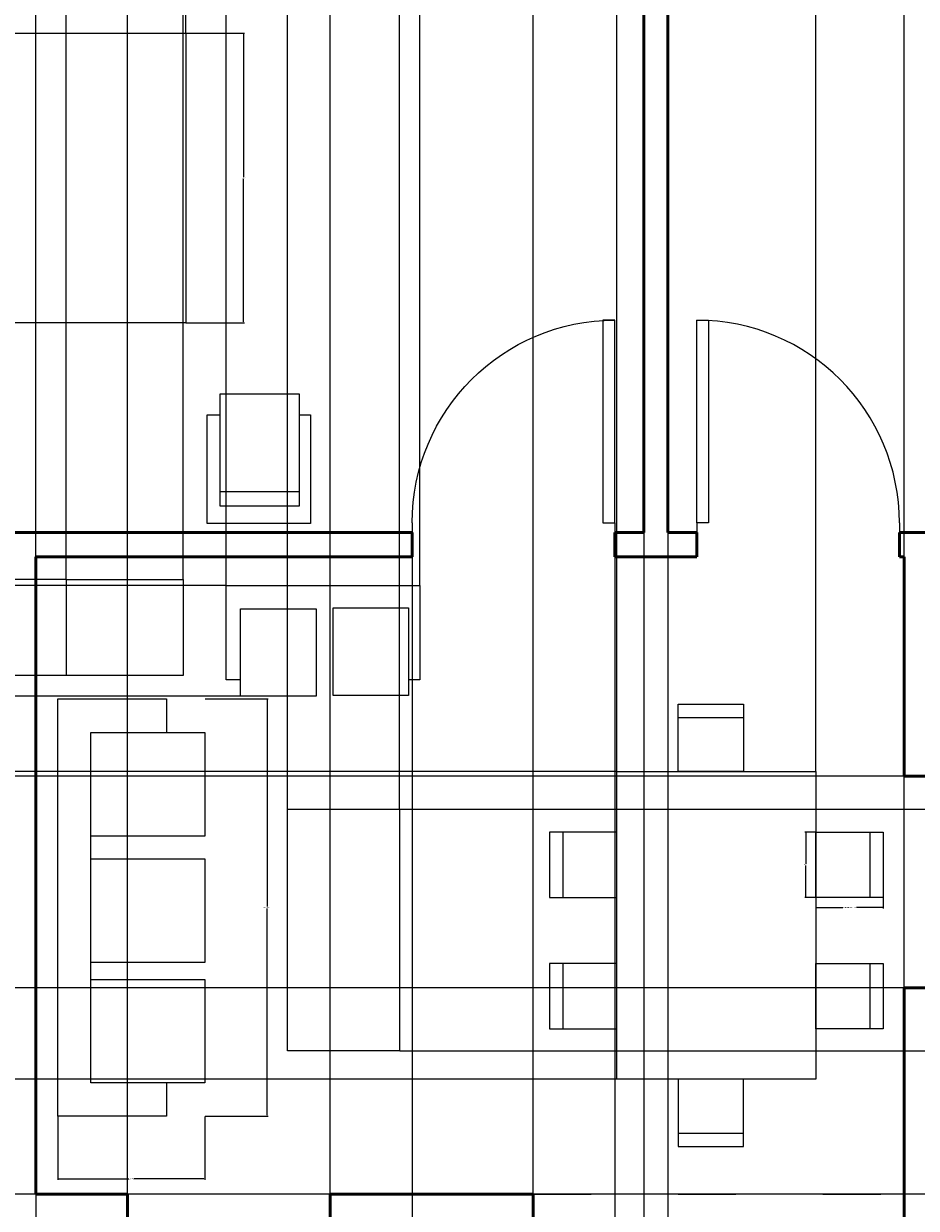
# Model space of a CAD drawing. Units: inches. Extents: x 115999 to 116502, y 188991 to 189729.
# Tile 3 of 5: x 116144 to 116329, y 189347 to 189592. Entities that reach past the tile are written whole.
import ezdxf

# ---------------------------------------------------------------- set-up
doc = ezdxf.new("R2010")
doc.units = ezdxf.units.IN
doc.linetypes.add('ACAD_ISO02W100', pattern=[15, 12, -3])
doc.linetypes.add('ACAD_ISO03W100', pattern=[30, 12, -18])
for name, color, linetype, lineweight in [('A-ANNO-DIMS', 2, 'Continuous', 18), ('A-DOOR', 4, 'Continuous', 25), ('A-FURN', 8, 'Continuous', 18), ('A-WALL', 7, 'Continuous', 50), ('A-WALL-OPEN', 7, 'ACAD_ISO03W100', 18), ('A-WALL-OVHD', 7, 'ACAD_ISO02W100', 18)]:
    doc.layers.add(name, color=color, linetype=linetype, lineweight=lineweight)
doc.styles.get("Standard").update_dxf_attribs({"font": 'arial.ttf'})
doc.dimstyles.get("Standard").update_dxf_attribs({"dimtxt": 0.18, "dimasz": 0.18, "dimexe": 0.18, "dimexo": 0.0625, "dimgap": 0.09, "dimtad": 0, "dimtih": 1, "dimtoh": 1, "dimdec": 4, "dimzin": 0, "dimdsep": 46, "dimtxsty": 'Standard', "dimcen": 0.09, "dimadec": 0, "dimazin": 0, "dimtfac": 1, "dimtdec": 4, "dimtofl": 0, "dimtmove": 0, "dimatfit": 3, "dimfxl": 1, "dimtolj": 1, "dimtzin": 0, "dimarcsym": 0})

# ---------------------------------------------------------------- blocks, each defined once
blk = doc.blocks.new('*U3')
for p, q in [((0, 0), (0, -5)), ((30, 0), (30, -5))]:
    blk.add_line(p, q)
blk.add_lwpolyline([(0, 0), (0, 30), (1.75, 30), (1.75, 0)], close=True)
blk.add_arc((0, 0), 30, 0, 90)
blk = doc.blocks.new('Bed - Queen')
for p, q in [((0, -80.00003), (0, 0)), ((0, 0), (59.99999, 0)), ((59.99999, 0), (59.99999, -80.00003)), ((7.99999, -1.2), (28.79998, -1.2)), ((7.99999, -14.4), (7.99999, -1.2)), ((28.79998, -1.2), (28.79998, -14.4)), ((31.19999, -1.2), (51.99999, -1.2)), ((31.19999, -14.4), (31.19999, -1.2)), ((51.99999, -1.2), (51.99999, -16.4)), ((0, -14.4), (44.8, -14.4)), ((59.99999, -29.6), (44.8, -14.4)), ((44.8, -14.4), (44.8, -29.6)), ((44.8, -16.8), (0, -16.8)), ((51.99999, -16.4), (46.79936, -16.4)), ((44.8, -29.6), (59.99999, -29.6)), ((59.99999, -80.00003), (0, -80.00003))]:
    blk.add_line(p, q)
blk = doc.blocks.new('SOFA-3-SEAT')
for points in [[(22.47, 6.88), (22.47, 0), (0, 0), (0, 86.44), (22.47, 86.44), (22.47, 79.43)], [(29.89, 6.88), (6.84, 6.88), (6.84, 79.43), (29.89, 79.43)]]:
    blk.add_lwpolyline(points)
for points in [[(30.42, 57.99), (6.84, 57.99), (6.84, 79.43), (30.42, 79.43)], [(30.42, 31.86), (6.84, 31.86), (6.84, 53.3), (30.42, 53.3)], [(30.42, 6.88), (6.84, 6.88), (6.84, 28.33), (30.42, 28.33)]]:
    blk.add_lwpolyline(points, close=True)
blk = doc.blocks.new('CHAIR-DINING')
blk.add_line((0, 11.19), (13.53, 11.19))
blk.add_lwpolyline([(0, 13.95), (13.53, 13.95), (13.53, 0), (0, 0)], close=True)
blk = doc.blocks.new('CHAIR-ARM')
blk.add_line((2.71, 6.64), (19.06, 6.64))
blk.add_lwpolyline([(2.71, 26.84), (19.06, 26.84), (19.06, 3.59), (2.71, 3.59)], close=True)
blk.add_lwpolyline([(19.06, 22.51), (21.46, 22.51), (21.46, 0), (0, 0), (0, 22.51), (2.71, 22.51)])
blk = doc.blocks.new('*D15')
at = {"layer": 'A-ANNO-DIMS', "color": 0, "lineweight": -2, "transparency": 16777216}
for p, q in [((116307.76, 189411.34), (116307.76, 189409.13)), ((116307.94, 189409.31), (116313.31, 189409.31)), ((116321.53, 189409.31), (116316.16, 189409.31)), ((116321.71, 189411.34), (116321.71, 189409.13))]:
    blk.add_line(p, q, dxfattribs=at)
at = {"layer": 'A-ANNO-DIMS', "color": 0, "transparency": 16777216}
for points in [[(116307.94, 189409.34), (116307.94, 189409.28), (116307.76, 189409.31)], [(116321.53, 189409.34), (116321.53, 189409.28), (116321.71, 189409.31)]]:
    blk.add_solid(points, dxfattribs=at)
at = {"layer": 'Defpoints', "color": 0, "transparency": 16777216}
for p in [(116307.76, 189411.41), (116321.71, 189411.41), (116321.71, 189409.31)]:
    blk.add_point(p, dxfattribs=at)
at = {"layer": 'A-ANNO-DIMS', "color": 0, "transparency": 16777216, "insert": (116314.74, 189409.31), "char_height": 0.18, "attachment_point": 5}
blk.add_mtext('\\A1;DINING CHAIR 14 TYP.', dxfattribs=at)
blk = doc.blocks.new('*D16')
at = {"layer": 'A-ANNO-DIMS', "color": 0, "lineweight": -2, "transparency": 16777216}
for p, q in [((116307.7, 189424.94), (116305.49, 189424.94)), ((116305.67, 189424.76), (116305.67, 189418.35)), ((116305.67, 189411.59), (116305.67, 189417.99)), ((116307.7, 189411.41), (116305.49, 189411.41))]:
    blk.add_line(p, q, dxfattribs=at)
at = {"layer": 'A-ANNO-DIMS', "color": 0, "transparency": 16777216}
for points in [[(116305.64, 189424.76), (116305.7, 189424.76), (116305.67, 189424.94)], [(116305.64, 189411.59), (116305.7, 189411.59), (116305.67, 189411.41)]]:
    blk.add_solid(points, dxfattribs=at)
at = {"layer": 'Defpoints', "color": 0, "transparency": 16777216}
for p in [(116307.76, 189424.94), (116305.67, 189411.41), (116307.76, 189411.41)]:
    blk.add_point(p, dxfattribs=at)
at = {"layer": 'A-ANNO-DIMS', "color": 0, "transparency": 16777216, "insert": (116305.67, 189418.17), "char_height": 0.18, "attachment_point": 5}
blk.add_mtext('\\A1;14 TYP.', dxfattribs=at)
blk = doc.blocks.new('*D21')
at = {"layer": 'A-ANNO-DIMS', "color": 0, "lineweight": -2, "transparency": 16777216}
for p, q in [((116097.14, 189590.46), (116097.14, 189602.58)), ((116097.32, 189602.4), (116135.84, 189602.4)), ((116176.96, 189602.4), (116138.45, 189602.4)), ((116177.14, 189590.46), (116177.14, 189602.58))]:
    blk.add_line(p, q, dxfattribs=at)
at = {"layer": 'A-ANNO-DIMS', "color": 0, "transparency": 16777216}
for points in [[(116097.32, 189602.43), (116097.32, 189602.37), (116097.14, 189602.4)], [(116176.96, 189602.43), (116176.96, 189602.37), (116177.14, 189602.4)]]:
    blk.add_solid(points, dxfattribs=at)
at = {"layer": 'Defpoints', "color": 0, "transparency": 16777216}
for p in [(116097.14, 189602.4), (116097.14, 189590.4), (116177.14, 189590.4)]:
    blk.add_point(p, dxfattribs=at)
at = {"layer": 'A-ANNO-DIMS', "color": 0, "transparency": 16777216, "insert": (116137.14, 189602.4), "char_height": 0.18, "attachment_point": 5}
blk.add_mtext('\\A1;QUEEN BED 80 TYP.', dxfattribs=at)
blk = doc.blocks.new('*D22')
at = {"layer": 'A-ANNO-DIMS', "color": 0, "lineweight": -2, "transparency": 16777216}
for p, q in [((116177.2, 189590.4), (116189.32, 189590.4)), ((116189.14, 189590.22), (116189.14, 189560.58)), ((116189.14, 189530.58), (116189.14, 189560.22)), ((116177.2, 189530.4), (116189.32, 189530.4))]:
    blk.add_line(p, q, dxfattribs=at)
at = {"layer": 'A-ANNO-DIMS', "color": 0, "transparency": 16777216}
for points in [[(116189.11, 189590.22), (116189.17, 189590.22), (116189.14, 189590.4)], [(116189.11, 189530.58), (116189.17, 189530.58), (116189.14, 189530.4)]]:
    blk.add_solid(points, dxfattribs=at)
at = {"layer": 'Defpoints', "color": 0, "transparency": 16777216}
for p in [(116177.14, 189590.4), (116189.14, 189590.4), (116177.14, 189530.4)]:
    blk.add_point(p, dxfattribs=at)
at = {"layer": 'A-ANNO-DIMS', "color": 0, "transparency": 16777216, "insert": (116189.14, 189560.4), "char_height": 0.18, "attachment_point": 5}
blk.add_mtext('\\A1;60 TYP.', dxfattribs=at)
blk = doc.blocks.new('*D25')
at = {"layer": 'A-ANNO-DIMS', "color": 0, "lineweight": -2, "transparency": 16777216}
for p, q in [((116181.15, 189452.53), (116194.23, 189452.53)), ((116194.05, 189452.35), (116194.05, 189409.49)), ((116194.05, 189366.27), (116194.05, 189409.13)), ((116181.15, 189366.09), (116194.23, 189366.09))]:
    blk.add_line(p, q, dxfattribs=at)
at = {"layer": 'A-ANNO-DIMS', "color": 0, "transparency": 16777216}
for points in [[(116194.02, 189452.35), (116194.08, 189452.35), (116194.05, 189452.53)], [(116194.02, 189366.27), (116194.08, 189366.27), (116194.05, 189366.09)]]:
    blk.add_solid(points, dxfattribs=at)
at = {"layer": 'Defpoints', "color": 0, "transparency": 16777216}
for p in [(116181.08, 189452.53), (116194.05, 189452.53), (116181.08, 189366.09)]:
    blk.add_point(p, dxfattribs=at)
at = {"layer": 'A-ANNO-DIMS', "color": 0, "transparency": 16777216, "insert": (116194.05, 189409.31), "char_height": 0.18, "attachment_point": 5}
blk.add_mtext('\\A1;SOFA 86 TYP.', dxfattribs=at)
blk = doc.blocks.new('*D26')
at = {"layer": 'A-ANNO-DIMS', "color": 0, "lineweight": -2, "transparency": 16777216}
for p, q in [((116150.66, 189366.03), (116150.66, 189352.94)), ((116181.08, 189366.03), (116181.08, 189352.94)), ((116150.84, 189353.12), (116165.34, 189353.12)), ((116180.9, 189353.12), (116166.4, 189353.12))]:
    blk.add_line(p, q, dxfattribs=at)
at = {"layer": 'A-ANNO-DIMS', "color": 0, "transparency": 16777216}
for points in [[(116150.84, 189353.15), (116150.84, 189353.09), (116150.66, 189353.12)], [(116180.9, 189353.15), (116180.9, 189353.09), (116181.08, 189353.12)]]:
    blk.add_solid(points, dxfattribs=at)
at = {"layer": 'Defpoints', "color": 0, "transparency": 16777216}
for p in [(116150.66, 189366.09), (116181.08, 189366.09), (116181.08, 189353.12)]:
    blk.add_point(p, dxfattribs=at)
at = {"layer": 'A-ANNO-DIMS', "color": 0, "transparency": 16777216, "insert": (116165.87, 189353.12), "char_height": 0.18, "attachment_point": 5}
blk.add_mtext('\\A1;30 TYP.', dxfattribs=at)
blk = doc.blocks.new('*D33')
at = {"layer": 'A-ANNO-DIMS', "color": 0, "lineweight": -2, "transparency": 16777216}
for p, q in [((116088.06, 189088.01), (116088.06, 189728.73)), ((116088.24, 189728.55), (116277.77, 189728.55)), ((116467.88, 189728.55), (116278.35, 189728.55)), ((116468.06, 189088.01), (116468.06, 189728.73))]:
    blk.add_line(p, q, dxfattribs=at)
at = {"layer": 'A-ANNO-DIMS', "color": 0, "transparency": 16777216}
for points in [[(116088.24, 189728.58), (116088.24, 189728.52), (116088.06, 189728.55)], [(116467.88, 189728.58), (116467.88, 189728.52), (116468.06, 189728.55)]]:
    blk.add_solid(points, dxfattribs=at)
at = {"layer": 'Defpoints', "color": 0, "transparency": 16777216}
for p in [(116468.06, 189728.55), (116088.06, 189087.95), (116468.06, 189087.95)]:
    blk.add_point(p, dxfattribs=at)
at = {"layer": 'A-ANNO-DIMS', "color": 0, "transparency": 16777216, "insert": (116278.06, 189728.55), "char_height": 0.18, "attachment_point": 5}
blk.add_mtext('\\A1;380', dxfattribs=at)
blk = doc.blocks.new('*D43')
at = {"layer": 'A-ANNO-DIMS', "color": 0, "lineweight": -2, "transparency": 16777216}
for p, q in [((116093.06, 189624.88), (116093.06, 188991.26)), ((116272.06, 189624.88), (116272.06, 188991.26)), ((116093.24, 188991.44), (116182.28, 188991.44)), ((116271.88, 188991.44), (116182.84, 188991.44))]:
    blk.add_line(p, q, dxfattribs=at)
at = {"layer": 'A-ANNO-DIMS', "color": 0, "transparency": 16777216}
for points in [[(116093.24, 188991.47), (116093.24, 188991.41), (116093.06, 188991.44)], [(116271.88, 188991.47), (116271.88, 188991.41), (116272.06, 188991.44)]]:
    blk.add_solid(points, dxfattribs=at)
at = {"layer": 'Defpoints', "color": 0, "transparency": 16777216}
for p in [(116093.06, 189624.95), (116272.06, 189624.95), (116272.06, 188991.44)]:
    blk.add_point(p, dxfattribs=at)
at = {"layer": 'A-ANNO-DIMS', "color": 0, "transparency": 16777216, "insert": (116182.56, 188991.44), "char_height": 0.18, "attachment_point": 5}
blk.add_mtext('\\A1;179', dxfattribs=at)
blk = doc.blocks.new('*D44')
at = {"layer": 'A-ANNO-DIMS', "color": 0, "lineweight": -2, "transparency": 16777216}
for p, q in [((116277.06, 189624.88), (116277.06, 188991.26)), ((116463.06, 189624.88), (116463.06, 188991.26)), ((116277.24, 188991.44), (116369.78, 188991.44)), ((116462.88, 188991.44), (116370.34, 188991.44))]:
    blk.add_line(p, q, dxfattribs=at)
at = {"layer": 'A-ANNO-DIMS', "color": 0, "transparency": 16777216}
for points in [[(116277.24, 188991.47), (116277.24, 188991.41), (116277.06, 188991.44)], [(116462.88, 188991.47), (116462.88, 188991.41), (116463.06, 188991.44)]]:
    blk.add_solid(points, dxfattribs=at)
at = {"layer": 'Defpoints', "color": 0, "transparency": 16777216}
for p in [(116277.06, 189624.95), (116463.06, 189624.95), (116463.06, 188991.44)]:
    blk.add_point(p, dxfattribs=at)
at = {"layer": 'A-ANNO-DIMS', "color": 0, "transparency": 16777216, "insert": (116370.06, 188991.44), "char_height": 0.18, "attachment_point": 5}
blk.add_mtext('\\A1;186', dxfattribs=at)
blk = doc.blocks.new('*D45')
at = {"layer": 'A-ANNO-DIMS', "color": 0, "lineweight": -2, "transparency": 16777216}
for p, q in [((116272.06, 189624.88), (116272.06, 188991.26)), ((116277.06, 189624.88), (116277.06, 188991.26)), ((116272.24, 188991.44), (116274.41, 188991.44)), ((116276.88, 188991.44), (116274.71, 188991.44))]:
    blk.add_line(p, q, dxfattribs=at)
at = {"layer": 'A-ANNO-DIMS', "color": 0, "transparency": 16777216}
for points in [[(116272.24, 188991.47), (116272.24, 188991.41), (116272.06, 188991.44)], [(116276.88, 188991.47), (116276.88, 188991.41), (116277.06, 188991.44)]]:
    blk.add_solid(points, dxfattribs=at)
at = {"layer": 'Defpoints', "color": 0, "transparency": 16777216}
for p in [(116272.06, 189624.95), (116277.06, 189624.95), (116277.06, 188991.44)]:
    blk.add_point(p, dxfattribs=at)
at = {"layer": 'A-ANNO-DIMS', "color": 0, "transparency": 16777216, "insert": (116274.56, 188991.44), "char_height": 0.18, "attachment_point": 5}
blk.add_mtext('\\A1;5', dxfattribs=at)
blk = doc.blocks.new('*D46')
at = {"layer": 'A-ANNO-DIMS', "color": 0, "lineweight": -2, "transparency": 16777216}
for p, q in [((116224.06, 189486.88), (116224.06, 188991.26)), ((116266.06, 189486.88), (116266.06, 188991.26)), ((116224.24, 188991.44), (116244.84, 188991.44)), ((116265.88, 188991.44), (116245.28, 188991.44))]:
    blk.add_line(p, q, dxfattribs=at)
at = {"layer": 'A-ANNO-DIMS', "color": 0, "transparency": 16777216}
for points in [[(116224.24, 188991.47), (116224.24, 188991.41), (116224.06, 188991.44)], [(116265.88, 188991.47), (116265.88, 188991.41), (116266.06, 188991.44)]]:
    blk.add_solid(points, dxfattribs=at)
at = {"layer": 'Defpoints', "color": 0, "transparency": 16777216}
for p in [(116224.06, 189486.95), (116266.06, 189486.95), (116266.06, 188991.44)]:
    blk.add_point(p, dxfattribs=at)
at = {"layer": 'A-ANNO-DIMS', "color": 0, "transparency": 16777216, "insert": (116245.06, 188991.44), "char_height": 0.18, "attachment_point": 5}
blk.add_mtext('\\A1;42', dxfattribs=at)
blk = doc.blocks.new('*D47')
at = {"layer": 'A-ANNO-DIMS', "color": 0, "lineweight": -2, "transparency": 16777216}
for p, q in [((116266.063078, 189486.884428), (116266.063078, 188991.259265)), ((116272.063078, 189486.884428), (116272.063078, 188991.259265)), ((116266.243078, 188991.439265), (116268.913651, 188991.439265)), ((116271.883078, 188991.439265), (116269.212505, 188991.439265))]:
    blk.add_line(p, q, dxfattribs=at)
at = {"layer": 'A-ANNO-DIMS', "color": 0, "transparency": 16777216}
for points in [[(116266.243078, 188991.469265), (116266.243078, 188991.409265), (116266.063078, 188991.439265)], [(116271.883078, 188991.469265), (116271.883078, 188991.409265), (116272.063078, 188991.439265)]]:
    blk.add_solid(points, dxfattribs=at)
at = {"layer": 'Defpoints', "color": 0, "transparency": 16777216}
for p in [(116266.063078, 189486.946928), (116272.063078, 189486.946928), (116272.063078, 188991.439265)]:
    blk.add_point(p, dxfattribs=at)
at = {"layer": 'A-ANNO-DIMS', "color": 0, "transparency": 16777216, "insert": (116269.063078, 188991.439265), "char_height": 0.18, "attachment_point": 5}
blk.add_mtext('\\A1;6', dxfattribs=at)
blk = doc.blocks.new('*D50')
at = {"layer": 'A-ANNO-DIMS', "color": 0, "lineweight": -2, "transparency": 16777216}
for p, q in [((116146.06, 189349.88), (116146.06, 188991.26)), ((116326.06, 189349.88), (116326.06, 188991.26)), ((116146.24, 188991.44), (116235.78, 188991.44)), ((116325.88, 188991.44), (116236.34, 188991.44))]:
    blk.add_line(p, q, dxfattribs=at)
at = {"layer": 'A-ANNO-DIMS', "color": 0, "transparency": 16777216}
for points in [[(116146.24, 188991.47), (116146.24, 188991.41), (116146.06, 188991.44)], [(116325.88, 188991.47), (116325.88, 188991.41), (116326.06, 188991.44)]]:
    blk.add_solid(points, dxfattribs=at)
at = {"layer": 'Defpoints', "color": 0, "transparency": 16777216}
for p in [(116146.06, 189349.95), (116326.06, 189349.95), (116326.06, 188991.44)]:
    blk.add_point(p, dxfattribs=at)
at = {"layer": 'A-ANNO-DIMS', "color": 0, "transparency": 16777216, "insert": (116236.06, 188991.44), "char_height": 0.18, "attachment_point": 5}
blk.add_mtext('\\A1;180', dxfattribs=at)
blk = doc.blocks.new('*D53')
at = {"layer": 'A-ANNO-DIMS', "color": 0, "lineweight": -2, "transparency": 16777216}
for p, q in [((116331, 189436.5), (115999.04, 189436.5)), ((115999.22, 189436.32), (115999.22, 189414.77)), ((115999.22, 189392.85), (115999.22, 189414.41)), ((116331, 189392.67), (115999.04, 189392.67))]:
    blk.add_line(p, q, dxfattribs=at)
at = {"layer": 'A-ANNO-DIMS', "color": 0, "transparency": 16777216}
for points in [[(115999.19, 189436.32), (115999.25, 189436.32), (115999.22, 189436.5)], [(115999.19, 189392.85), (115999.25, 189392.85), (115999.22, 189392.67)]]:
    blk.add_solid(points, dxfattribs=at)
at = {"layer": 'Defpoints', "color": 0, "transparency": 16777216}
for p in [(115999.22, 189436.5), (116331.06, 189436.5), (116331.06, 189392.67)]:
    blk.add_point(p, dxfattribs=at)
at = {"layer": 'A-ANNO-DIMS', "color": 0, "transparency": 16777216, "insert": (115999.22, 189414.59), "char_height": 0.18, "attachment_point": 5}
blk.add_mtext('\\A1;43.83', dxfattribs=at)
blk = doc.blocks.new('*D54')
at = {"layer": 'A-ANNO-DIMS', "color": 0, "lineweight": -2, "transparency": 16777216}
for p, q in [((116266.5, 189437.51), (116266.5, 189728.73)), ((116266.68, 189728.55), (116286.73, 189728.55)), ((116307.58, 189728.55), (116287.53, 189728.55)), ((116307.76, 189437.51), (116307.76, 189728.73))]:
    blk.add_line(p, q, dxfattribs=at)
at = {"layer": 'A-ANNO-DIMS', "color": 0, "transparency": 16777216}
for points in [[(116266.68, 189728.58), (116266.68, 189728.52), (116266.5, 189728.55)], [(116307.58, 189728.58), (116307.58, 189728.52), (116307.76, 189728.55)]]:
    blk.add_solid(points, dxfattribs=at)
at = {"layer": 'Defpoints', "color": 0, "transparency": 16777216}
for p in [(116307.76, 189728.55), (116266.5, 189437.45), (116307.76, 189437.45)]:
    blk.add_point(p, dxfattribs=at)
at = {"layer": 'A-ANNO-DIMS', "color": 0, "transparency": 16777216, "insert": (116287.13, 189728.55), "char_height": 0.18, "attachment_point": 5}
blk.add_mtext('\\A1;41.26', dxfattribs=at)
blk = doc.blocks.new('*D55')
at = {"layer": 'A-ANNO-DIMS', "color": 0, "lineweight": -2, "transparency": 16777216}
for p, q in [((116266.44, 189437.45), (115999.04, 189437.45)), ((115999.22, 189437.27), (115999.22, 189405.79)), ((115999.22, 189373.95), (115999.22, 189405.43)), ((116266.44, 189373.77), (115999.04, 189373.77))]:
    blk.add_line(p, q, dxfattribs=at)
at = {"layer": 'A-ANNO-DIMS', "color": 0, "transparency": 16777216}
for points in [[(115999.19, 189437.27), (115999.25, 189437.27), (115999.22, 189437.45)], [(115999.19, 189373.95), (115999.25, 189373.95), (115999.22, 189373.77)]]:
    blk.add_solid(points, dxfattribs=at)
at = {"layer": 'Defpoints', "color": 0, "transparency": 16777216}
for p in [(115999.22, 189437.45), (116266.5, 189437.45), (116266.5, 189373.77)]:
    blk.add_point(p, dxfattribs=at)
at = {"layer": 'A-ANNO-DIMS', "color": 0, "transparency": 16777216, "insert": (115999.22, 189405.61), "char_height": 0.18, "attachment_point": 5}
blk.add_mtext('\\A1;63.68', dxfattribs=at)
blk = doc.blocks.new('*D67')
at = {"layer": 'A-ANNO-DIMS', "color": 0, "lineweight": -2, "transparency": 16777216}
for p, q in [((116331, 189392.67), (115999.04, 189392.67)), ((115999.22, 189392.49), (115999.22, 189371.49)), ((115999.22, 189350.13), (115999.22, 189371.13)), ((116331, 189349.95), (115999.04, 189349.95))]:
    blk.add_line(p, q, dxfattribs=at)
at = {"layer": 'A-ANNO-DIMS', "color": 0, "transparency": 16777216}
for points in [[(115999.19, 189392.49), (115999.25, 189392.49), (115999.22, 189392.67)], [(115999.19, 189350.13), (115999.25, 189350.13), (115999.22, 189349.95)]]:
    blk.add_solid(points, dxfattribs=at)
at = {"layer": 'Defpoints', "color": 0, "transparency": 16777216}
for p in [(115999.22, 189392.67), (116331.06, 189392.67), (116331.06, 189349.95)]:
    blk.add_point(p, dxfattribs=at)
at = {"layer": 'A-ANNO-DIMS', "color": 0, "transparency": 16777216, "insert": (115999.22, 189371.31), "char_height": 0.18, "attachment_point": 5}
blk.add_mtext('\\A1;42.73', dxfattribs=at)
blk = doc.blocks.new('*D71')
at = {"layer": 'A-ANNO-DIMS', "color": 0, "lineweight": -2, "transparency": 16777216}
for p, q in [((116165.06, 189350.01), (116165.06, 189728.73)), ((116165.24, 189728.55), (116185.84, 189728.55)), ((116206.88, 189728.55), (116186.28, 189728.55)), ((116207.06, 189350.01), (116207.06, 189728.73))]:
    blk.add_line(p, q, dxfattribs=at)
at = {"layer": 'A-ANNO-DIMS', "color": 0, "transparency": 16777216}
for points in [[(116165.24, 189728.58), (116165.24, 189728.52), (116165.06, 189728.55)], [(116206.88, 189728.58), (116206.88, 189728.52), (116207.06, 189728.55)]]:
    blk.add_solid(points, dxfattribs=at)
at = {"layer": 'Defpoints', "color": 0, "transparency": 16777216}
for p in [(116207.06, 189728.55), (116165.06, 189349.95), (116207.06, 189349.95)]:
    blk.add_point(p, dxfattribs=at)
at = {"layer": 'A-ANNO-DIMS', "color": 0, "transparency": 16777216, "insert": (116186.06, 189728.55), "char_height": 0.18, "attachment_point": 5}
blk.add_mtext('\\A1;42', dxfattribs=at)
blk = doc.blocks.new('*D72')
at = {"layer": 'A-ANNO-DIMS', "color": 0, "lineweight": -2, "transparency": 16777216}
for p, q in [((116249.18, 189350.01), (116249.18, 189728.73)), ((116249.36, 189728.55), (116287.23, 189728.55)), ((116325.88, 189728.55), (116288.02, 189728.55)), ((116326.06, 189350.01), (116326.06, 189728.73))]:
    blk.add_line(p, q, dxfattribs=at)
at = {"layer": 'A-ANNO-DIMS', "color": 0, "transparency": 16777216}
for points in [[(116249.36, 189728.58), (116249.36, 189728.52), (116249.18, 189728.55)], [(116325.88, 189728.58), (116325.88, 189728.52), (116326.06, 189728.55)]]:
    blk.add_solid(points, dxfattribs=at)
at = {"layer": 'Defpoints', "color": 0, "transparency": 16777216}
for p in [(116326.06, 189728.55), (116249.18, 189349.95), (116326.06, 189349.95)]:
    blk.add_point(p, dxfattribs=at)
at = {"layer": 'A-ANNO-DIMS', "color": 0, "transparency": 16777216, "insert": (116287.62, 189728.55), "char_height": 0.18, "attachment_point": 5}
blk.add_mtext('\\A1;76.88', dxfattribs=at)
blk = doc.blocks.new('*D74')
at = {"layer": 'A-ANNO-DIMS', "color": 0, "lineweight": -2, "transparency": 16777216}
for p, q in [((116146.06, 189350.01), (116146.06, 189728.73)), ((116146.24, 189728.55), (116155.35, 189728.55)), ((116164.88, 189728.55), (116155.77, 189728.55)), ((116165.06, 189350.01), (116165.06, 189728.73))]:
    blk.add_line(p, q, dxfattribs=at)
at = {"layer": 'A-ANNO-DIMS', "color": 0, "transparency": 16777216}
for points in [[(116146.24, 189728.58), (116146.24, 189728.52), (116146.06, 189728.55)], [(116164.88, 189728.58), (116164.88, 189728.52), (116165.06, 189728.55)]]:
    blk.add_solid(points, dxfattribs=at)
at = {"layer": 'Defpoints', "color": 0, "transparency": 16777216}
for p in [(116165.06, 189728.55), (116146.06, 189349.95), (116165.06, 189349.95)]:
    blk.add_point(p, dxfattribs=at)
at = {"layer": 'A-ANNO-DIMS', "color": 0, "transparency": 16777216, "insert": (116155.56, 189728.55), "char_height": 0.18, "attachment_point": 5}
blk.add_mtext('\\A1;19', dxfattribs=at)
blk = doc.blocks.new('*D78')
at = {"layer": 'A-ANNO-DIMS', "color": 0, "lineweight": -2, "transparency": 16777216}
for p, q in [((116198.25, 189429.74), (116198.25, 189728.73)), ((116198.43, 189728.55), (116209.47, 189728.55)), ((116221.29, 189728.55), (116210.25, 189728.55)), ((116221.47, 189429.74), (116221.47, 189728.73))]:
    blk.add_line(p, q, dxfattribs=at)
at = {"layer": 'A-ANNO-DIMS', "color": 0, "transparency": 16777216}
for points in [[(116198.43, 189728.58), (116198.43, 189728.52), (116198.25, 189728.55)], [(116221.29, 189728.58), (116221.29, 189728.52), (116221.47, 189728.55)]]:
    blk.add_solid(points, dxfattribs=at)
at = {"layer": 'Defpoints', "color": 0, "transparency": 16777216}
for p in [(116221.47, 189728.55), (116198.25, 189429.68), (116221.47, 189429.68)]:
    blk.add_point(p, dxfattribs=at)
at = {"layer": 'A-ANNO-DIMS', "color": 0, "transparency": 16777216, "insert": (116209.86, 189728.55), "char_height": 0.18, "attachment_point": 5}
blk.add_mtext('\\A1;23.22', dxfattribs=at)
blk = doc.blocks.new('*D79')
at = {"layer": 'A-ANNO-DIMS', "color": 0, "lineweight": -2, "transparency": 16777216}
for p, q in [((116221.53, 189429.68), (116501.84, 189429.68)), ((116501.66, 189429.5), (116501.66, 189404.83)), ((116501.66, 189379.81), (116501.66, 189404.47)), ((116221.53, 189379.63), (116501.84, 189379.63))]:
    blk.add_line(p, q, dxfattribs=at)
at = {"layer": 'A-ANNO-DIMS', "color": 0, "transparency": 16777216}
for points in [[(116501.63, 189429.5), (116501.69, 189429.5), (116501.66, 189429.68)], [(116501.63, 189379.81), (116501.69, 189379.81), (116501.66, 189379.63)]]:
    blk.add_solid(points, dxfattribs=at)
at = {"layer": 'Defpoints', "color": 0, "transparency": 16777216}
for p in [(116221.47, 189429.68), (116501.66, 189429.68), (116221.47, 189379.63)]:
    blk.add_point(p, dxfattribs=at)
at = {"layer": 'A-ANNO-DIMS', "color": 0, "transparency": 16777216, "insert": (116501.66, 189404.65), "char_height": 0.18, "attachment_point": 5}
blk.add_mtext('\\A1;50.05', dxfattribs=at)
blk = doc.blocks.new('*D80')
at = {"layer": 'A-ANNO-DIMS', "color": 0, "lineweight": -2, "transparency": 16777216}
for p, q in [((116185.52, 189476.05), (116185.52, 189728.73)), ((116185.7, 189728.55), (116205.21, 189728.55)), ((116225.51, 189728.55), (116206, 189728.55)), ((116225.69, 189476.05), (116225.69, 189728.73))]:
    blk.add_line(p, q, dxfattribs=at)
at = {"layer": 'A-ANNO-DIMS', "color": 0, "transparency": 16777216}
for points in [[(116185.7, 189728.58), (116185.7, 189728.52), (116185.52, 189728.55)], [(116225.51, 189728.58), (116225.51, 189728.52), (116225.69, 189728.55)]]:
    blk.add_solid(points, dxfattribs=at)
at = {"layer": 'Defpoints', "color": 0, "transparency": 16777216}
for p in [(116225.69, 189728.55), (116185.52, 189475.99), (116225.69, 189475.99)]:
    blk.add_point(p, dxfattribs=at)
at = {"layer": 'A-ANNO-DIMS', "color": 0, "transparency": 16777216, "insert": (116205.6, 189728.55), "char_height": 0.18, "attachment_point": 5}
blk.add_mtext('\\A1;40.17', dxfattribs=at)
blk = doc.blocks.new('*D81')
at = {"layer": 'A-ANNO-DIMS', "color": 0, "lineweight": -2, "transparency": 16777216}
for p, q in [((116185.46, 189475.99), (115999.04, 189475.99)), ((115999.22, 189475.81), (115999.22, 189464.71)), ((115999.22, 189453.24), (115999.22, 189464.34)), ((116188.46, 189453.06), (115999.04, 189453.06))]:
    blk.add_line(p, q, dxfattribs=at)
at = {"layer": 'A-ANNO-DIMS', "color": 0, "transparency": 16777216}
for points in [[(115999.19, 189475.81), (115999.25, 189475.81), (115999.22, 189475.99)], [(115999.19, 189453.24), (115999.25, 189453.24), (115999.22, 189453.06)]]:
    blk.add_solid(points, dxfattribs=at)
at = {"layer": 'Defpoints', "color": 0, "transparency": 16777216}
for p in [(116185.52, 189475.99), (115999.22, 189453.06), (116188.52, 189453.06)]:
    blk.add_point(p, dxfattribs=at)
at = {"layer": 'A-ANNO-DIMS', "color": 0, "transparency": 16777216, "insert": (115999.22, 189464.52), "char_height": 0.18, "attachment_point": 5}
blk.add_mtext('\\A1;22.926', dxfattribs=at)
blk = doc.blocks.new('*D82')
at = {"layer": 'A-ANNO-DIMS', "color": 0, "lineweight": -2, "transparency": 16777216}
for p, q in [((116152.4, 189477.27), (116152.4, 189728.73)), ((116152.58, 189728.55), (116164.04, 189728.55)), ((116176.43, 189728.55), (116164.97, 189728.55)), ((116176.61, 189477.27), (116176.61, 189728.73))]:
    blk.add_line(p, q, dxfattribs=at)
at = {"layer": 'A-ANNO-DIMS', "color": 0, "transparency": 16777216}
for points in [[(116152.58, 189728.58), (116152.58, 189728.52), (116152.4, 189728.55)], [(116176.43, 189728.58), (116176.43, 189728.52), (116176.61, 189728.55)]]:
    blk.add_solid(points, dxfattribs=at)
at = {"layer": 'Defpoints', "color": 0, "transparency": 16777216}
for p in [(116176.61, 189728.55), (116152.4, 189477.21), (116176.61, 189477.21)]:
    blk.add_point(p, dxfattribs=at)
at = {"layer": 'A-ANNO-DIMS', "color": 0, "transparency": 16777216, "insert": (116164.51, 189728.55), "char_height": 0.18, "attachment_point": 5}
blk.add_mtext('\\A1;24.204', dxfattribs=at)
blk = doc.blocks.new('*D83')
at = {"layer": 'A-ANNO-DIMS', "color": 0, "lineweight": -2, "transparency": 16777216}
for p, q in [((116152.34, 189477.21), (115999.04, 189477.21)), ((115999.22, 189477.03), (115999.22, 189467.47)), ((115999.22, 189457.56), (115999.22, 189467.11)), ((116152.34, 189457.38), (115999.04, 189457.38))]:
    blk.add_line(p, q, dxfattribs=at)
at = {"layer": 'A-ANNO-DIMS', "color": 0, "transparency": 16777216}
for points in [[(115999.19, 189477.03), (115999.25, 189477.03), (115999.22, 189477.21)], [(115999.19, 189457.56), (115999.25, 189457.56), (115999.22, 189457.38)]]:
    blk.add_solid(points, dxfattribs=at)
at = {"layer": 'Defpoints', "color": 0, "transparency": 16777216}
for p in [(115999.22, 189477.21), (116152.4, 189477.21), (116152.4, 189457.38)]:
    blk.add_point(p, dxfattribs=at)
at = {"layer": 'A-ANNO-DIMS', "color": 0, "transparency": 16777216, "insert": (115999.22, 189467.29), "char_height": 0.18, "attachment_point": 5}
blk.add_mtext('\\A1;19.83', dxfattribs=at)

msp = doc.modelspace()

# ---------------------------------------------------------------- linework, layer by layer
at = {"layer": 'A-FURN'}
for points in [[(116152.4048, 189477.2058), (116176.6085, 189477.2058), (116176.6085, 189457.376), (116152.4048, 189457.376)], [(116188.5186, 189471.1941), (116204.1981, 189471.1941), (116204.1981, 189453.0603), (116188.5186, 189453.0603)], [(116207.6703, 189471.3815), (116223.3498, 189471.3815), (116223.3498, 189453.2476), (116207.6703, 189453.2476)], [(116266.5001, 189437.4482), (116307.7598, 189437.4482), (116307.7598, 189373.7675), (116266.5001, 189373.7675)], [(116198.2486, 189429.6768), (116221.4703, 189429.6768), (116221.4703, 189379.6257), (116198.2486, 189379.6257)]]:
    msp.add_lwpolyline(points, close=True, dxfattribs=at)
for points in [[(116188.5186, 189456.4441), (116185.5193, 189456.4441), (116185.5193, 189475.9866), (116225.6867, 189475.9866), (116225.6867, 189456.4441)], [(116225.6867, 189456.4441), (116223.3498, 189456.4441)]]:
    msp.add_lwpolyline(points, dxfattribs=at)
at = {"layer": 'A-WALL'}
for p, q in [((116272.0631, 189624.9469), (116272.0631, 189486.9469)), ((116277.0631, 189624.9469), (116277.0631, 189486.9469)), ((116093.0631, 189486.9469), (116224.0631, 189486.9469)), ((116224.0631, 189486.9469), (116224.0631, 189481.9469)), ((116266.0631, 189486.9469), (116266.0631, 189481.9469)), ((116266.0631, 189486.9469), (116272.0631, 189486.9469)), ((116277.0631, 189486.9469), (116283.0631, 189486.9469)), ((116283.0631, 189486.9469), (116283.0631, 189481.9469)), ((116325.0631, 189486.9469), (116325.0631, 189481.9469)), ((116325.0631, 189486.9469), (116463.0631, 189486.9469)), ((116146.0631, 189481.9469), (116146.0631, 189349.9469)), ((116146.0631, 189481.9469), (116224.0631, 189481.9469)), ((116266.0631, 189481.9469), (116283.0631, 189481.9469)), ((116277.0631, 189481.9469), (116283.0631, 189481.9469)), ((116325.0631, 189481.9469), (116326.0631, 189481.9469)), ((116325.0631, 189481.9469), (116326.0631, 189481.9469)), ((116326.0631, 189481.9469), (116326.0631, 189436.5016)), ((116326.0631, 189436.5016), (116331.0631, 189436.5016)), ((116326.0631, 189392.6745), (116331.0631, 189392.6745)), ((116326.0631, 189392.6745), (116326.0631, 189344.9469)), ((116146.0631, 189349.9469), (116165.0631, 189349.9469)), ((116165.0631, 189344.9469), (116165.0631, 189349.9469)), ((116207.0631, 189344.9469), (116207.0631, 189349.9469)), ((116207.0631, 189349.9469), (116249.1823, 189349.9469)), ((116249.1823, 189344.9469), (116249.1823, 189349.9469))]:
    msp.add_line(p, q, dxfattribs=at)
at = {"layer": 'A-WALL-OPEN'}
msp.add_line((116249.1823, 189349.9469), (116326.0631, 189349.9469), dxfattribs=at)
at = {"layer": 'A-WALL-OVHD'}
msp.add_line((116326.0631, 189392.6745), (116326.0631, 189436.5016), dxfattribs=at)

# ---------------------------------------------------------------- block references
at = {"layer": 'A-DOOR', "yscale": 1.400000000000193, "zscale": 1.400000000000193}
for p, xscale in [((116266.0631, 189488.9469), -1.400000000000193), ((116283.0631, 189488.9469), 1.400000000000193)]:
    msp.add_blockref('*U3', p, dxfattribs=dict(at, xscale=xscale))
at = {"layer": 'A-DOOR', "xscale": 1.400000000000193, "yscale": 1.400000000000193, "zscale": 1.400000000000193, "rotation": 180}
msp.add_blockref('*U3', (116207.0631, 189342.9469), dxfattribs=at)
at = {"layer": 'A-FURN'}
for name, p, rotation in [('Bed - Queen', (116097.142, 189530.3971), 90), ('CHAIR-DINING', (116307.7598, 189424.94), 269.9999999998937), ('CHAIR-DINING', (116307.7598, 189397.7046), 269.9999999998937)]:
    msp.add_blockref(name, p, dxfattribs=dict(at, rotation=rotation))
for name, p in [('CHAIR-ARM', (116181.5682, 189488.8569)), ('SOFA-3-SEAT', (116150.6627, 189366.0896)), ('CHAIR-DINING', (116279.2191, 189437.4482))]:
    msp.add_blockref(name, p, dxfattribs=at)
at = {"layer": 'A-FURN', "extrusion": (0, 0, -1), "zscale": -1}
for p, rotation in [((-116266.5001, 189424.94), 269.9999999998937), ((-116266.5001, 189397.7046), 269.9999999998937), ((-116279.2191, 189373.7675), 180)]:
    msp.add_blockref('CHAIR-DINING', p, dxfattribs=dict(at, rotation=rotation))

# ---------------------------------------------------------------- dimensions: what is measured, and where the dimension line sits
at = {"layer": 'A-ANNO-DIMS'}
for base, p1, p2, override, picture, middle in [((116468.0631, 189728.5469), (116088.0631, 189087.9469), (116468.0631, 189087.9469), {"dimdec": 0, "dimlfac": 1, "dimrnd": 0, "dimzin": 0, "dimdsep": 46, "dimlunit": 2}, '*D33', (116278.0631, 189728.5469)), ((116165.0631, 189728.5469), (116146.0631, 189349.9469), (116165.0631, 189349.9469), {"dimdec": 0, "dimlfac": 1, "dimrnd": 0, "dimzin": 0, "dimdsep": 46, "dimlunit": 2}, '*D74', (116155.5631, 189728.5469)), ((116176.6085, 189728.5469), (116152.4048, 189477.2058), (116176.6085, 189477.2058), {"dimdec": 3, "dimlfac": 1, "dimrnd": 0, "dimzin": 0, "dimdsep": 46, "dimlunit": 2}, '*D82', (116164.5066, 189728.5469)), ((116207.0631, 189728.5469), (116165.0631, 189349.9469), (116207.0631, 189349.9469), {"dimdec": 0, "dimlfac": 1, "dimrnd": 0, "dimzin": 0, "dimdsep": 46, "dimlunit": 2}, '*D71', (116186.0631, 189728.5469)), ((116225.6867, 189728.5469), (116185.5193, 189475.9866), (116225.6867, 189475.9866), {"dimdec": 2, "dimlfac": 1, "dimrnd": 0, "dimzin": 0, "dimdsep": 46, "dimlunit": 2}, '*D80', (116205.603, 189728.5469)), ((116221.4703, 189728.5469), (116198.2486, 189429.6768), (116221.4703, 189429.6768), {"dimdec": 2, "dimlfac": 1, "dimrnd": 0, "dimzin": 0, "dimdsep": 46, "dimlunit": 2}, '*D78', (116209.8595, 189728.5469)), ((116326.0631, 189728.5469), (116249.1823, 189349.9469), (116326.0631, 189349.9469), {"dimdec": 2, "dimlfac": 1, "dimrnd": 0, "dimzin": 0, "dimdsep": 46, "dimlunit": 2}, '*D72', (116287.6227, 189728.5469)), ((116307.7598, 189728.5469), (116266.5001, 189437.4482), (116307.7598, 189437.4482), {"dimdec": 2, "dimlfac": 1, "dimrnd": 0, "dimzin": 0, "dimdsep": 46, "dimlunit": 2}, '*D54', (116287.13, 189728.5469)), ((116272.0631, 188991.4393), (116093.0631, 189624.9469), (116272.0631, 189624.9469), {"dimdec": 0, "dimlfac": 1, "dimrnd": 0, "dimzin": 0, "dimdsep": 46, "dimlunit": 2}, '*D43', (116182.5631, 188991.4393)), ((116277.0631, 188991.4393), (116272.0631, 189624.9469), (116277.0631, 189624.9469), {"dimdec": 0, "dimlfac": 1, "dimrnd": 0, "dimzin": 0, "dimdsep": 46, "dimlunit": 2}, '*D45', (116274.5631, 188991.4393)), ((116463.0631, 188991.4393), (116277.0631, 189624.9469), (116463.0631, 189624.9469), {"dimdec": 0, "dimlfac": 1, "dimrnd": 0, "dimzin": 0, "dimdsep": 46, "dimlunit": 2}, '*D44', (116370.0631, 188991.4393)), ((116266.0631, 188991.4393), (116224.0631, 189486.9469), (116266.0631, 189486.9469), {"dimdec": 0, "dimlfac": 1, "dimrnd": 0, "dimzin": 0, "dimdsep": 46, "dimlunit": 2}, '*D46', (116245.0631, 188991.4393)), ((116272.0631, 188991.4393), (116266.0631, 189486.9469), (116272.0631, 189486.9469), {"dimdec": 0, "dimlfac": 1, "dimrnd": 0, "dimzin": 0, "dimdsep": 46, "dimlunit": 2}, '*D47', (116269.0631, 188991.4393)), ((116326.0631, 188991.4393), (116146.0631, 189349.9469), (116326.0631, 189349.9469), {"dimdec": 0, "dimlfac": 1, "dimrnd": 0, "dimzin": 0, "dimdsep": 46, "dimlunit": 2}, '*D50', (116236.0631, 188991.4393))]:
    dim = msp.add_linear_dim(base=base, p1=p1, p2=p2, dimstyle='Standard', override=override, dxfattribs=at)
    dim.commit()
    dim.dimension.update_dxf_attribs({"geometry": picture, "text_midpoint": middle})
for base, p1, p2, angle, text, picture, middle in [((116097.142, 189602.3971), (116177.1421, 189590.397), (116097.142, 189590.397), 180, 'QUEEN BED <> TYP.', '*D21', (116137.142, 189602.3971)), ((116189.1421, 189590.397), (116177.1421, 189530.3971), (116177.1421, 189590.397), 90, '<> TYP.', '*D22', (116189.1421, 189560.3971)), ((116194.049, 189452.5309), (116181.0828, 189366.0896), (116181.0828, 189452.5309), 90, 'SOFA <> TYP.', '*D25', (116194.049, 189409.3103)), ((116305.6666, 189411.407), (116307.7598, 189424.94), (116307.7598, 189411.407), 270, '<> TYP.', '*D16', (116305.6666, 189418.1735))]:
    dim = msp.add_linear_dim(base=base, p1=p1, p2=p2, angle=angle, text=text, dimstyle='Standard', override={"dimdec": 0, "dimlfac": 1, "dimrnd": 0, "dimzin": 0, "dimdsep": 46, "dimlunit": 2}, dxfattribs=at)
    dim.commit()
    dim.dimension.update_dxf_attribs({"geometry": picture, "text_midpoint": middle})
for base, p1, p2, override, picture, middle in [((115999.2211, 189453.0603), (116185.5193, 189475.9866), (116188.5186, 189453.0603), {"dimdec": 3, "dimlfac": 1, "dimrnd": 0, "dimzin": 0, "dimdsep": 46, "dimlunit": 2}, '*D81', (115999.2211, 189464.5234)), ((115999.2211, 189477.2058), (116152.4048, 189457.376), (116152.4048, 189477.2058), {"dimdec": 2, "dimlfac": 1, "dimrnd": 0, "dimzin": 0, "dimdsep": 46, "dimlunit": 2}, '*D83', (115999.2211, 189467.2909)), ((115999.2211, 189437.4482), (116266.5001, 189373.7675), (116266.5001, 189437.4482), {"dimdec": 2, "dimlfac": 1, "dimrnd": 0, "dimzin": 0, "dimdsep": 46, "dimlunit": 2}, '*D55', (115999.2211, 189405.6079)), ((115999.2211, 189436.5016), (116331.0631, 189392.6745), (116331.0631, 189436.5016), {"dimdec": 2, "dimlfac": 1, "dimrnd": 0, "dimzin": 0, "dimdsep": 46, "dimlunit": 2}, '*D53', (115999.2211, 189414.588)), ((116501.6631, 189429.6768), (116221.4703, 189379.6257), (116221.4703, 189429.6768), {"dimdec": 2, "dimlfac": 1, "dimrnd": 0, "dimzin": 0, "dimdsep": 46, "dimlunit": 2}, '*D79', (116501.6631, 189404.6513)), ((115999.2211, 189392.6745), (116331.0631, 189349.9469), (116331.0631, 189392.6745), {"dimdec": 2, "dimlfac": 1, "dimrnd": 0, "dimzin": 0, "dimdsep": 46, "dimlunit": 2}, '*D67', (115999.2211, 189371.3107))]:
    dim = msp.add_linear_dim(base=base, p1=p1, p2=p2, angle=90, dimstyle='Standard', override=override, dxfattribs=at)
    dim.commit()
    dim.dimension.update_dxf_attribs({"geometry": picture, "text_midpoint": middle})
for base, p1, p2, text, picture, middle in [((116321.7142, 189409.3138), (116307.7598, 189411.407), (116321.7142, 189411.407), 'DINING CHAIR <> TYP.', '*D15', (116314.737, 189409.3138)), ((116181.0828, 189353.1235), (116150.6627, 189366.0896), (116181.0828, 189366.0896), '<> TYP.', '*D26', (116165.8728, 189353.1235))]:
    dim = msp.add_linear_dim(base=base, p1=p1, p2=p2, text=text, dimstyle='Standard', override={"dimdec": 0, "dimlfac": 1, "dimrnd": 0, "dimzin": 0, "dimdsep": 46, "dimlunit": 2}, dxfattribs=at)
    dim.commit()
    dim.dimension.update_dxf_attribs({"geometry": picture, "text_midpoint": middle})

doc.saveas('drawing.dxf')
